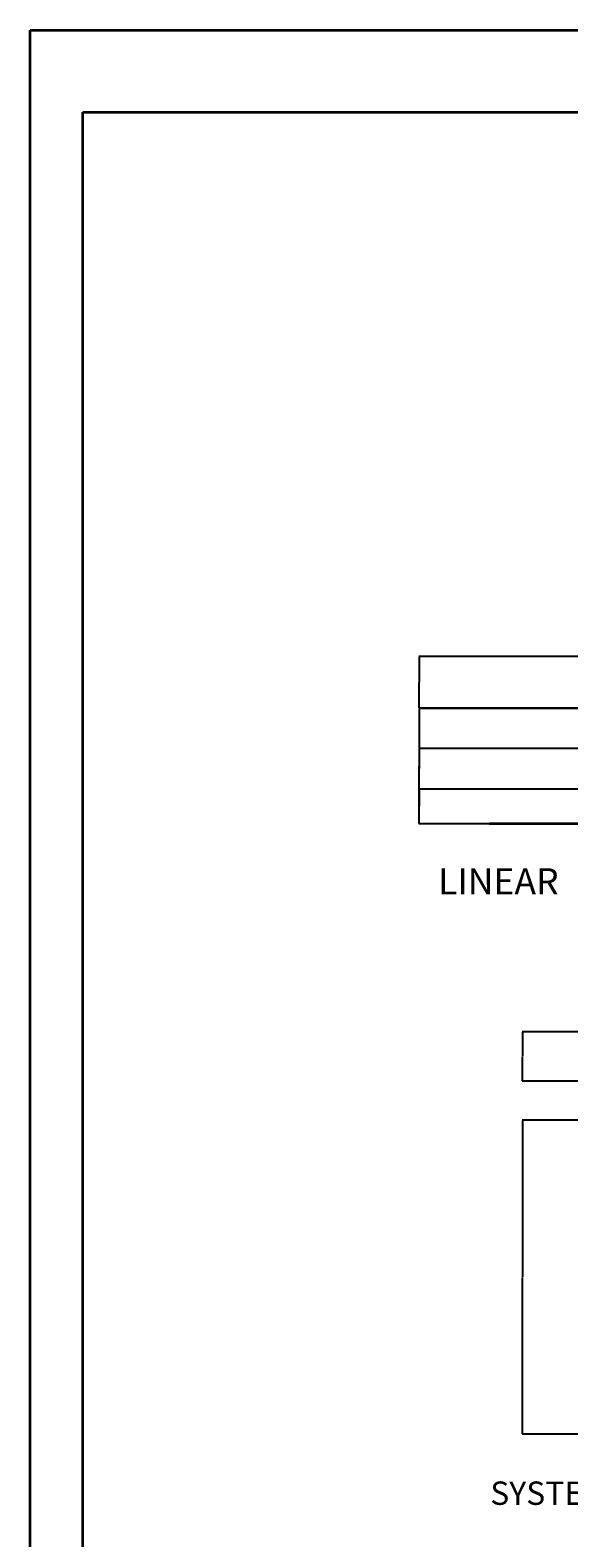
# Model space of a CAD drawing. Units: inches. Extents: x -934 to 898, y -1502 to 444.
# Tile 5 of 10: x -934 to -511, y -739 to 444. Entities that reach past the tile are written whole.
import ezdxf

# ---------------------------------------------------------------- set-up
doc = ezdxf.new("R2010")
doc.units = ezdxf.units.IN
doc.header["$MEASUREMENT"] = 0
for name, color, linetype, lineweight in [('A-ANNO-DIMS', 2, 'Continuous', 18), ('A-ANNO-TITL', 7, 'Continuous', 30), ('A-ANNO-TTLB', 7, 'Continuous', 35), ('L-GRND', 7, 'Continuous', 35)]:
    doc.layers.add(name, color=color, linetype=linetype, lineweight=lineweight)
doc.styles.get("Standard").update_dxf_attribs({"font": 'arial.ttf'})
doc.dimstyles.get("Standard").update_dxf_attribs({"dimtxt": 0.18, "dimasz": 0.18, "dimexe": 0.18, "dimexo": 0.0625, "dimgap": 0.09, "dimtad": 0, "dimtih": 1, "dimtoh": 1, "dimdec": 4, "dimzin": 0, "dimdsep": 46, "dimtxsty": 'Standard', "dimcen": 0.09, "dimadec": 0, "dimazin": 0, "dimtfac": 1, "dimtdec": 4, "dimtofl": 0, "dimtmove": 0, "dimatfit": 3, "dimfxl": 1, "dimtolj": 1, "dimtzin": 0, "dimarcsym": 0})

# ---------------------------------------------------------------- blocks, each defined once
blk = doc.blocks.new('*D84')
at = {"layer": 'A-ANNO-DIMS', "color": 0, "lineweight": -2, "transparency": 16777216}
for p, q in [((-423, -88.2), (-628.5, -88.2)), ((-628.4, -88.4), (-628.4, -133.3)), ((-628.4, -178.5), (-628.4, -133.6)), ((-423.3, -178.7), (-628.5, -178.7))]:
    blk.add_line(p, q, dxfattribs=at)
at = {"layer": 'A-ANNO-DIMS', "color": 0, "transparency": 16777216}
for points in [[(-628.4, -88.4), (-628.3, -88.4), (-628.4, -88.2)], [(-628.4, -178.5), (-628.3, -178.5), (-628.4, -178.7)]]:
    blk.add_solid(points, dxfattribs=at)
at = {"layer": 'Defpoints', "color": 0, "transparency": 16777216}
for p in [(-628.4, -88.2), (-422.9, -88.2), (-423.3, -178.7)]:
    blk.add_point(p, dxfattribs=at)
at = {"layer": 'A-ANNO-DIMS', "color": 0, "transparency": 16777216, "insert": (-628.4, -133.5), "char_height": 0.18, "attachment_point": 5}
blk.add_mtext('\\A1;90.45', dxfattribs=at)
blk = doc.blocks.new('*D85')
at = {"layer": 'A-ANNO-DIMS', "color": 0, "lineweight": -2, "transparency": 16777216}
for p, q in [((-397.9, -47.4), (-628.5, -47.4)), ((-628.4, -47.5), (-628.4, -67.5)), ((-628.4, -87.8), (-628.4, -67.9)), ((-398, -88), (-628.5, -88))]:
    blk.add_line(p, q, dxfattribs=at)
at = {"layer": 'A-ANNO-DIMS', "color": 0, "transparency": 16777216}
for points in [[(-628.4, -47.5), (-628.3, -47.5), (-628.4, -47.4)], [(-628.4, -87.8), (-628.3, -87.8), (-628.4, -88)]]:
    blk.add_solid(points, dxfattribs=at)
at = {"layer": 'Defpoints', "color": 0, "transparency": 16777216}
for p in [(-628.4, -47.4), (-397.8, -47.4), (-397.9, -88)]:
    blk.add_point(p, dxfattribs=at)
at = {"layer": 'A-ANNO-DIMS', "color": 0, "transparency": 16777216, "insert": (-628.4, -67.7), "char_height": 0.18, "attachment_point": 5}
blk.add_mtext('\\A1;40.63', dxfattribs=at)
blk = doc.blocks.new('*D95')
at = {"layer": 'A-ANNO-DIMS', "color": 0, "lineweight": -2, "transparency": 16777216}
for p, q in [((-351.6, -151.5), (-628.5, -151.5)), ((-628.4, -151.7), (-628.4, -164.9)), ((-628.4, -178.5), (-628.4, -165.3)), ((-351.6, -178.7), (-628.5, -178.7))]:
    blk.add_line(p, q, dxfattribs=at)
at = {"layer": 'A-ANNO-DIMS', "color": 0, "transparency": 16777216}
for points in [[(-628.4, -151.7), (-628.3, -151.7), (-628.4, -151.5)], [(-628.4, -178.5), (-628.3, -178.5), (-628.4, -178.7)]]:
    blk.add_solid(points, dxfattribs=at)
at = {"layer": 'Defpoints', "color": 0, "transparency": 16777216}
for p in [(-628.4, -151.5), (-351.6, -151.5), (-351.6, -178.7)]:
    blk.add_point(p, dxfattribs=at)
at = {"layer": 'A-ANNO-DIMS', "color": 0, "transparency": 16777216, "insert": (-628.4, -165.1), "char_height": 0.18, "attachment_point": 5}
blk.add_mtext('\\A1;27.16', dxfattribs=at)
blk = doc.blocks.new('*D96')
at = {"layer": 'A-ANNO-DIMS', "color": 0, "lineweight": -2, "transparency": 16777216}
for p, q in [((-351.6, -119.6), (-628.5, -119.6)), ((-628.4, -119.8), (-628.4, -135.4)), ((-628.4, -151.3), (-628.4, -135.8)), ((-351.6, -151.5), (-628.5, -151.5))]:
    blk.add_line(p, q, dxfattribs=at)
at = {"layer": 'A-ANNO-DIMS', "color": 0, "transparency": 16777216}
for points in [[(-628.4, -119.8), (-628.3, -119.8), (-628.4, -119.6)], [(-628.4, -151.3), (-628.3, -151.3), (-628.4, -151.5)]]:
    blk.add_solid(points, dxfattribs=at)
at = {"layer": 'Defpoints', "color": 0, "transparency": 16777216}
for p in [(-628.4, -119.6), (-351.6, -119.6), (-351.6, -151.5)]:
    blk.add_point(p, dxfattribs=at)
at = {"layer": 'A-ANNO-DIMS', "color": 0, "transparency": 16777216, "insert": (-628.4, -135.6), "char_height": 0.18, "attachment_point": 5}
blk.add_mtext('\\A1;31.89', dxfattribs=at)
blk = doc.blocks.new('*D105')
at = {"layer": 'A-ANNO-DIMS', "color": 0, "lineweight": -2, "transparency": 16777216}
for p, q in [((-366.9, -411.5), (-547.4, -411.5)), ((-547.2, -411.7), (-547.2, -534.6)), ((-547.2, -657.8), (-547.2, -534.9)), ((-349.5, -658), (-547.4, -658))]:
    blk.add_line(p, q, dxfattribs=at)
at = {"layer": 'A-ANNO-DIMS', "color": 0, "transparency": 16777216}
for points in [[(-547.2, -411.7), (-547.2, -411.7), (-547.2, -411.5)], [(-547.2, -657.8), (-547.2, -657.8), (-547.2, -658)]]:
    blk.add_solid(points, dxfattribs=at)
at = {"layer": 'Defpoints', "color": 0, "transparency": 16777216}
for p in [(-547.2, -411.5), (-366.8, -411.5), (-349.4, -658)]:
    blk.add_point(p, dxfattribs=at)
at = {"layer": 'A-ANNO-DIMS', "color": 0, "transparency": 16777216, "insert": (-547.2, -534.7), "char_height": 0.18, "attachment_point": 5}
blk.add_mtext('\\A1;246.5', dxfattribs=at)
blk = doc.blocks.new('*D106')
at = {"layer": 'A-ANNO-DIMS', "color": 0, "lineweight": -2, "transparency": 16777216}
for p, q in [((58.1, -342.1), (-547.4, -342.1)), ((-547.2, -342.3), (-547.2, -361.3)), ((-547.2, -380.6), (-547.2, -361.6)), ((-216.2, -380.8), (-547.4, -380.8))]:
    blk.add_line(p, q, dxfattribs=at)
at = {"layer": 'A-ANNO-DIMS', "color": 0, "transparency": 16777216}
for points in [[(-547.2, -342.3), (-547.2, -342.3), (-547.2, -342.1)], [(-547.2, -380.6), (-547.2, -380.6), (-547.2, -380.8)]]:
    blk.add_solid(points, dxfattribs=at)
at = {"layer": 'Defpoints', "color": 0, "transparency": 16777216}
for p in [(-547.2, -342.1), (58.2, -342.1), (-216.1, -380.8)]:
    blk.add_point(p, dxfattribs=at)
at = {"layer": 'A-ANNO-DIMS', "color": 0, "transparency": 16777216, "insert": (-547.2, -361.4), "char_height": 0.18, "attachment_point": 5}
blk.add_mtext('\\A1;38.685', dxfattribs=at)

msp = doc.modelspace()

# ---------------------------------------------------------------- linework, layer by layer
at = {"layer": 'A-ANNO-TTLB'}
for points in [[(-933.5092, 444.4646), (897.7239, 444.4646), (897.7239, -1501.5858), (-933.5092, -1501.5858)], [(-892.081, 380.0228), (832.9871, 380.0228), (832.9871, -1448.0237), (-892.081, -1448.0237)]]:
    msp.add_lwpolyline(points, close=True, dxfattribs=at)
at = {"layer": 'L-GRND'}
msp.add_line((284.8904, -178.6804), (-573.1189, -178.6804), dxfattribs=at)

# ---------------------------------------------------------------- texts
at = {"layer": 'A-ANNO-TITL'}
for s, height, p in [('LINEAR   CAMPUS   AXIS ELEVATION   RESEARCH   AND   INNOVATION   SPINE ', 20.457511, (-613.4854, -234.1138)), ('SYSTEM   SECTION   CLIMATE   CONTROLLED   ATRIUM   AND FACADE   POD', 18.353224, (-572.4968, -713.5413))]:
    msp.add_text(s, height=height, dxfattribs=at).set_placement(p)

# ---------------------------------------------------------------- dimensions: what is measured, and where the dimension line sits
at = {"layer": 'A-ANNO-DIMS'}
for base, p1, p2, override, picture, middle in [((-628.3689, -47.3642), (-397.9256, -87.9953), (-397.7996, -47.3642), {"dimdec": 2, "dimlfac": 1, "dimrnd": 0, "dimzin": 0, "dimdsep": 46, "dimlunit": 2}, '*D85', (-628.3689, -67.6798)), ((-628.3689, -88.2276), (-423.2792, -178.6804), (-422.9344, -88.2276), {"dimdec": 2, "dimlfac": 1, "dimrnd": 0, "dimzin": 0, "dimdsep": 46, "dimlunit": 2}, '*D84', (-628.3689, -133.454)), ((-628.3689, -119.6248), (-351.5859, -151.5178), (-351.5859, -119.6248), {"dimdec": 2, "dimlfac": 1, "dimrnd": 0, "dimzin": 0, "dimdsep": 46, "dimlunit": 2}, '*D96', (-628.3689, -135.5713)), ((-628.3689, -151.5178), (-351.5859, -178.6804), (-351.5859, -151.5178), {"dimdec": 2, "dimlfac": 1, "dimrnd": 0, "dimzin": 0, "dimdsep": 46, "dimlunit": 2}, '*D95', (-628.3689, -165.0991)), ((-547.1946, -342.1018), (-216.1305, -380.7865), (58.1805, -342.1018), {"dimdec": 3, "dimlfac": 1, "dimrnd": 0, "dimzin": 0, "dimdsep": 46, "dimlunit": 2}, '*D106', (-547.1946, -361.4441)), ((-547.1946, -411.4835), (-349.4313, -658.003), (-366.8176, -411.4835), {"dimdec": 1, "dimlfac": 1, "dimrnd": 0, "dimzin": 0, "dimdsep": 46, "dimlunit": 2}, '*D105', (-547.1946, -534.7433))]:
    dim = msp.add_linear_dim(base=base, p1=p1, p2=p2, angle=90, dimstyle='Standard', override=override, dxfattribs=at)
    dim.commit()
    dim.dimension.update_dxf_attribs({"geometry": picture, "text_midpoint": middle})

doc.saveas('drawing.dxf')
